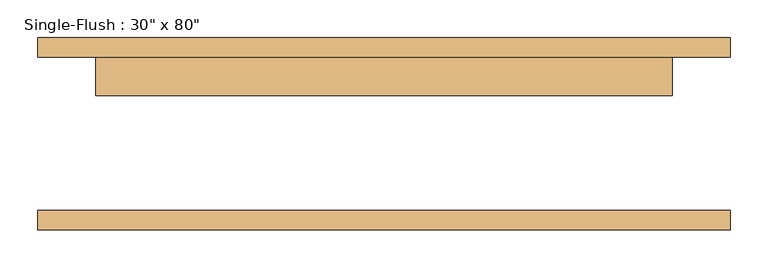
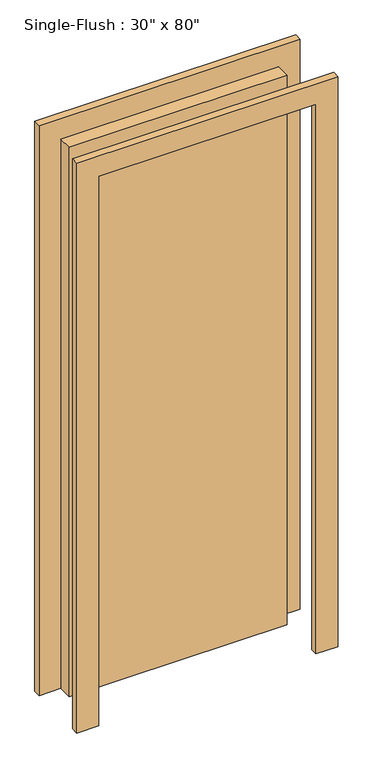
"""IFC4 building model written with IfcOpenShell, lengths in millimetres: door geometry."""

from ifc_helpers import new_model, si_unit, frame, origin, origin_with_axes, place, context, project, spatial, polyline, outline, extrude, source, transform, mapped, element, save


def door_fadea3f2(model_context):
    return source(origin(), model_context, "Body", "SweptSolid", [
        extrude(outline(polyline([(2108.2, -457.2), (0.0, -457.2), (0.0, -381.0), (2032.0, -381.0), (2032.0, 381.0), (0.0, 381.0), (0.0, 457.2), (2108.2, 457.2), (2108.2, -457.2)])), frame((0.0, 101.6, 0.0), z_axis=(0.0, 1.0, 0.0), x_axis=(0.0, 0.0, 1.0)), (0.0, 0.0, 1.0), 25.4),
        extrude(outline(polyline([(2108.2, 457.2), (2108.2, -457.2), (0.0, -457.2), (0.0, -381.0), (2032.0, -381.0), (2032.0, 381.0), (0.0, 381.0), (0.0, 457.2), (2108.2, 457.2)])), frame((0.0, -127.0, 0.0), z_axis=(0.0, 1.0, 0.0), x_axis=(0.0, 0.0, 1.0)), (0.0, 0.0, 1.0), 25.4),
        extrude(outline(polyline([(381.0, 50.8), (-381.0, 50.8), (-381.0, 101.6), (381.0, 101.6), (381.0, 50.8)])), origin_with_axes(), (0.0, 0.0, 1.0), 2032.0),
    ])


if __name__ == "__main__":
    model = new_model("IFC4")
    model_context = context("Model", 3, world=origin())
    ifc_project = project(units=[si_unit("LENGTHUNIT", "METRE", prefix="MILLI")], contexts=[model_context])
    site = spatial("IfcSite", under=ifc_project)
    building = spatial("IfcBuilding", under=site)
    placement = place(None, origin())
    door_shape = door_fadea3f2(model_context)
    element("IfcDoor", 1, ObjectType="Single-Flush : 30\" x 80\"", at=placement, inside=building, context=model_context, shape_type="MappedRepresentation", body=[
        mapped(door_shape, transform((0.0, 0.0, 0.0), x_axis=(1.0, 0.0, 0.0), y_axis=(0.0, 1.0, 0.0), z_axis=(0.0, 0.0, 1.0))),
    ])
    save(model, "model.ifc")

# Revit data of these elements
# Type "Single-Flush : 30\" x 80\""
#   Type Mark = "5"
#   Construction Type Id = "MDOOR"
#   Assembly Code = "C1020"
#   Analytic Construction = "Metal"
#   Thickness = 0' - 2"
#   Heat Transfer Coefficient (U) = 0.651978 BTU/(h·ft²·°F)
#   Height = 6' - 8"
#   Trim Projection Ext = 0' - 1"
#   Trim Projection Int = 0' - 1"
#   Trim Width = 0' - 3"
#   Width = 2' - 6"
#   Define Thermal Properties by = 1
#   Door Material = Door - Panel
#   Frame Material = Door - Frame
#   Visual Light Transmittance = 0
#   Solar Heat Gain Coefficient = 0
#   Function = (empty or 0)
#   Wall Closure = (empty or 0)
# Element 1 (IfcDoor, "Single-Flush : 30\" x 80\"")
#   Materials on its faces: "Door - Frame", "Door - Panel"
# Materials
#   "Door - Panel": class "Wood", colour RGB 210 159 95, transparency 0
#   "Door - Frame": colour RGB 118 70 51, transparency 0
